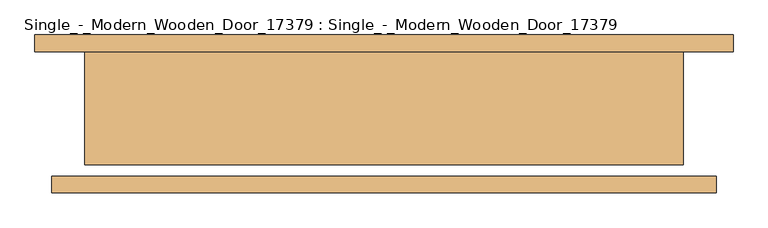
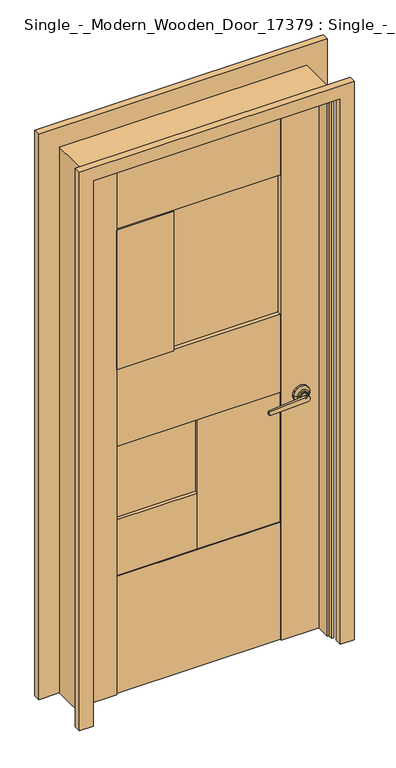
"""IFC4 building model written with IfcOpenShell, lengths in millimetres: door geometry, Single_-_Modern_Wooden_Door_17379 : Single_-_Modern_Wooden_Door_17379."""

from ifc_helpers import new_model, si_unit, point, frame, frame_2d, origin, origin_with_axes, place, context, project, spatial, polyline, circle_curve, ellipse_curve, trimmed, segment, composite_curve, outline, extrude, faceted_brep, source, transform, mapped, element, save
from ifc_brep_helpers import plane_surface, cylinder_surface, revolved_surface, advanced_brep


def single_modern_wooden_door_17379_single_modern_wooden_door_9761f21e(model_context):
    return source(origin(), model_context, "Body", "SolidModel", [
        extrude(outline(polyline([(2133.6, -457.2), (2133.6, 457.2), (0.0, 457.2), (0.0, 508.0), (2184.4, 508.0), (2184.4, -508.0), (0.0, -508.0), (0.0, -457.2), (2133.6, -457.2)])), frame((0.0, -139.7, 0.0), z_axis=(0.0, 1.0, 0.0), x_axis=(0.0, 0.0, 1.0)), (0.0, 0.0, 1.0), 25.4),
        advanced_brep(
        [(533.4, 76.2, 0.0), (457.2, 76.2, 0.0), (457.2, 88.9, 0.0), (479.425, 88.9, 0.0), (479.425, 95.25, 0.0), (485.775, 101.6, 0.0), (533.4, 101.6, 0.0), (533.4, 76.2, 2209.8), (-533.4, 76.2, 2209.8), (-533.4, 76.2, 0.0), (-457.2, 76.2, 0.0), (-457.2, 76.2, 2133.6), (457.2, 76.2, 2133.6), (457.2, 88.9, 2133.6), (-457.2, 88.9, 2133.6), (-457.2, 88.9, 0.0), (-479.425, 88.9, 0.0), (-479.425, 88.9, 2155.825), (479.425, 88.9, 2155.825), (479.425, 95.25, 2155.825), (485.775, 101.6, 2162.175), (-485.775, 101.6, 2162.175), (-485.775, 101.6, 0.0), (-533.4, 101.6, 0.0), (-533.4, 101.6, 2209.8), (533.4, 101.6, 2209.8), (-479.425, 95.25, 0.0), (-479.425, 95.25, 2155.825)],
        [
            (0, 1),
            (1, 2),
            (2, 3),
            (3, 4),
            (4, 5, circle_curve(frame((485.775, 95.25, 0.0), z_axis=(0.0, 0.0, -1.0), x_axis=(-1.0, 0.0, 0.0)), 6.35)),
            (5, 6),
            (6, 0),
            (0, 7),
            (7, 8),
            (8, 9),
            (9, 10),
            (10, 11),
            (11, 12),
            (12, 1),
            (12, 13),
            (13, 2),
            (13, 14),
            (14, 15),
            (15, 16),
            (16, 17),
            (17, 18),
            (18, 3),
            (18, 19),
            (19, 4),
            (19, 20, ellipse_curve(frame((485.775, 95.25, 2162.175), z_axis=(0.7071067811865457, 0.0, -0.7071067811865492), x_axis=(-0.7071067811865492, 0.0, -0.7071067811865458)), 8.9802561, 6.35)),
            (20, 5),
            (20, 21),
            (21, 22),
            (22, 23),
            (23, 24),
            (24, 25),
            (25, 6),
            (25, 7),
            (8, 24),
            (23, 9),
            (22, 26, circle_curve(frame((-485.775, 95.25, 0.0), z_axis=(0.0, 0.0, -1.0), x_axis=(1.0, 0.0, 0.0)), 6.35)),
            (26, 16),
            (15, 10),
            (14, 11),
            (27, 17),
            (26, 27),
            (21, 27, ellipse_curve(frame((-485.775, 95.25, 2162.175), z_axis=(-0.7071067811865492, 0.0, -0.7071067811865458), x_axis=(-0.7071067811865458, 0.0, 0.7071067811865492)), 8.9802561, 6.35)),
            (27, 19),
        ],
        [
            plane_surface(frame((457.2, 0.0, 0.0), z_axis=(0.0, 0.0, -1.0), x_axis=(0.0, -1.0, 0.0))),
            plane_surface(frame((533.4, 76.2, 0.0), z_axis=(0.0, -1.0, 0.0), x_axis=(0.0, 0.0, 1.0))),
            plane_surface(frame((457.2, 76.2, 0.0), z_axis=(-1.0, 0.0, 0.0), x_axis=(0.0, 0.0, 1.0))),
            plane_surface(frame((457.2, 88.9, 0.0), z_axis=(0.0, 1.0, 0.0), x_axis=(0.0, 0.0, 1.0))),
            plane_surface(frame((479.425, 88.9, 0.0), z_axis=(-1.0, 0.0, 0.0), x_axis=(0.0, 0.0, 1.0))),
            cylinder_surface(frame((485.775, 95.25, 0.0), z_axis=(0.0, 0.0, -1.0), x_axis=(-1.0, 0.0, 0.0)), 6.35),
            plane_surface(frame((485.775, 101.6, 0.0), z_axis=(0.0, 1.0, 0.0), x_axis=(0.0, 0.0, 1.0))),
            plane_surface(frame((533.4, 101.6, 0.0), z_axis=(1.0, 0.0, 0.0), x_axis=(0.0, 0.0, 1.0))),
            plane_surface(frame((-533.4, 101.6, 2209.8), z_axis=(-1.0, 0.0, 0.0), x_axis=(0.0, 0.0, -1.0))),
            plane_surface(frame((-457.2, 0.0, 0.0), z_axis=(0.0, 0.0, -1.0), x_axis=(0.0, -1.0, 0.0))),
            plane_surface(frame((-457.2, 76.2, 2133.6), z_axis=(1.0, 0.0, 0.0), x_axis=(0.0, 0.0, -1.0))),
            plane_surface(frame((-479.425, 88.9, 2155.825), z_axis=(1.0, 0.0, 0.0), x_axis=(0.0, 0.0, -1.0))),
            cylinder_surface(frame((-485.775, 95.25, 2133.6), z_axis=(0.0, 0.0, 1.0), x_axis=(1.0, 0.0, 0.0)), 6.35),
            plane_surface(frame((457.2, 76.2, 2133.6), z_axis=(0.0, 0.0, -1.0), x_axis=(-1.0, 0.0, 0.0))),
            plane_surface(frame((479.425, 88.9, 2155.825), z_axis=(0.0, 0.0, -1.0), x_axis=(-1.0, 0.0, 0.0))),
            cylinder_surface(frame((457.2, 95.25, 2162.175), z_axis=(1.0, 0.0, 0.0), x_axis=(0.0, 0.0, -1.0)), 6.35),
            plane_surface(frame((533.4, 101.6, 2209.8), z_axis=(0.0, 0.0, 1.0), x_axis=(-1.0, 0.0, 0.0))),
        ],
        [
            (0, [[1, 2, 3, 4, 5, 6, 7]]),
            (1, [[-1, 8, 9, 10, 11, 12, 13, 14]]),
            (2, [[-2, -14, 15, 16]]),
            (3, [[-3, -16, 17, 18, 19, 20, 21, 22]]),
            (4, [[-4, -22, 23, 24]]),
            (5, [[-5, -24, 25, 26]]),
            (6, [[-6, -26, 27, 28, 29, 30, 31, 32]]),
            (7, [[-7, -32, 33, -8]]),
            (8, [[34, -30, 35, -10]]),
            (9, [[-35, -29, 36, 37, -19, 38, -11]]),
            (10, [[39, -12, -38, -18]]),
            (11, [[40, -20, -37, 41]]),
            (12, [[42, -41, -36, -28]]),
            (13, [[-15, -13, -39, -17]]),
            (14, [[-23, -21, -40, 43]]),
            (15, [[-25, -43, -42, -27]]),
            (16, [[-33, -31, -34, -9]]),
        ],
    ),
        faceted_brep([(444.5, 76.2, 0.0), (457.2, 76.2, 0.0), (457.2, -96.9526688, 0.0), (449.8578125, -96.9526688, 0.0), (449.8578125, -78.3473783, 0.0), (444.5, -78.3473783, 0.0), (444.5, 76.2, 2120.9), (-444.5, 76.2, 2120.9), (-444.5, 76.2, 0.0), (-457.2, 76.2, 0.0), (-457.2, 76.2, 2133.6), (457.2, 76.2, 2133.6), (457.2, -96.9526688, 2133.6), (-457.2, -96.9526688, 2133.6), (-457.2, -96.9526688, 0.0), (-449.8578125, -96.9526688, 0.0), (-449.8578125, -96.9526688, 2126.2578125), (449.8578125, -96.9526688, 2126.2578125), (449.8578125, -78.3473783, 2126.2578125), (-449.8578125, -78.3473783, 2126.2578125), (-449.8578125, -78.3473783, 0.0), (-444.5, -78.3473783, 0.0), (-444.5, -78.3473783, 2120.9), (444.5, -78.3473783, 2120.9)], [[[0, 1, 2, 3, 4, 5]], [[1, 0, 6, 7, 8, 9, 10, 11]], [[2, 1, 11, 12]], [[3, 2, 12, 13, 14, 15, 16, 17]], [[4, 3, 17, 18]], [[5, 4, 18, 19, 20, 21, 22, 23]], [[0, 5, 23, 6]], [[7, 22, 21, 8]], [[8, 21, 20, 15, 14, 9]], [[13, 10, 9, 14]], [[19, 16, 15, 20]], [[12, 11, 10, 13]], [[6, 23, 22, 7]], [[18, 17, 16, 19]]]),
        extrude(outline(polyline([(-304.8, -25.4), (-444.5, -25.4), (-444.5, 25.4), (-304.8, 25.4), (-304.8, -25.4)])), origin_with_axes(), (0.0, 0.0, 1.0), 2120.9),
        extrude(outline(polyline([(444.5, -25.4), (304.8, -25.4), (304.8, 25.4), (444.5, 25.4), (444.5, -25.4)])), origin_with_axes(), (0.0, 0.0, 1.0), 2120.9),
        extrude(outline(polyline([(304.8, -19.05), (-304.8, -19.05), (-304.8, 19.05), (304.8, 19.05), (304.8, -19.05)])), frame((0.0, 0.0, 0.7183756), z_axis=(0.0, 0.0, 1.0), x_axis=(1.0, 0.0, 0.0)), (0.0, 0.0, 1.0), 457.2),
        extrude(outline(polyline([(304.8, -19.05), (-304.8, -19.05), (-304.8, 19.05), (304.8, 19.05), (304.8, -19.05)])), frame((0.0, 0.0, 965.6301148), z_axis=(0.0, 0.0, 1.0), x_axis=(1.0, 0.0, 0.0)), (0.0, 0.0, 1.0), 304.8),
        extrude(outline(polyline([(304.8, -19.05), (-304.8, -19.05), (-304.8, 19.05), (304.8, 19.05), (304.8, -19.05)])), frame((0.0, 0.0, 1816.1), z_axis=(0.0, 0.0, 1.0), x_axis=(1.0, 0.0, 0.0)), (0.0, 0.0, 1.0), 304.8),
        extrude(outline(polyline([(304.8, -2.7903573), (-304.8, -2.7903573), (-304.8, 3.5596427), (304.8, 3.5596427), (304.8, -2.7903573)])), frame((0.0, 0.0, 676.8253621), z_axis=(0.0, 0.0, 1.0), x_axis=(1.0, 0.0, 0.0)), (0.0, 0.0, 1.0), 1139.2746379),
        extrude(outline(polyline([(-93.0839177, -25.4), (-304.8, -25.4), (-304.8, 15.875), (-93.0839177, 15.875), (-93.0839177, -25.4)])), frame((0.0, 0.0, 1270.4301148), z_axis=(0.0, 0.0, 1.0), x_axis=(1.0, 0.0, 0.0)), (0.0, 0.0, 1.0), 545.6698852),
        extrude(outline(polyline([(304.8, -15.875), (0.0, -15.875), (0.0, 15.875), (304.8, 15.875), (304.8, -15.875)])), frame((0.0, 0.0, 457.9183756), z_axis=(0.0, 0.0, 1.0), x_axis=(1.0, 0.0, 0.0)), (0.0, 0.0, 1.0), 507.7117392),
        extrude(outline(polyline([(0.0, -15.875), (-304.8, -15.875), (-304.8, 15.875), (0.0, 15.875), (0.0, -15.875)])), frame((0.0, 0.0, 457.9183756), z_axis=(0.0, 0.0, 1.0), x_axis=(1.0, 0.0, 0.0)), (0.0, 0.0, 1.0), 218.9069865),
        advanced_brep(
        [(344.5942945, 33.3375, 944.6720157), (405.1016039, 33.3375, 944.6720157), (405.1016039, 26.9875, 944.6720157), (344.5942945, 26.9875, 944.6720157), (353.5745507, 42.3177561, 944.6720157), (396.1213477, 42.3177561, 944.6720157), (359.9245507, 42.3177561, 944.6720157), (389.7713477, 42.3177561, 944.6720157), (359.9245507, 48.6677561, 944.6720157), (389.7713477, 48.6677561, 944.6720157), (374.8479492, 48.6677561, 944.6720157), (374.8479492, 26.9875, 944.6720157)],
        [
            (0, 1, circle_curve(frame((374.8479492, 33.3375, 944.6720157), z_axis=(0.0, -1.0, 0.0), x_axis=(1.0, 0.0, 0.0)), 30.2536547)),
            (1, 2),
            (2, 3, circle_curve(frame((374.8479492, 26.9875, 944.6720157), z_axis=(0.0, 1.0, 0.0), x_axis=(1.0, 0.0, 0.0)), 30.2536547)),
            (3, 0),
            (1, 0, circle_curve(frame((374.8479492, 33.3375, 944.6720157), z_axis=(0.0, -1.0, 0.0), x_axis=(1.0, 0.0, 0.0)), 30.2536547)),
            (3, 2, circle_curve(frame((374.8479492, 26.9875, 944.6720157), z_axis=(0.0, 1.0, 0.0), x_axis=(1.0, 0.0, 0.0)), 30.2536547)),
            (4, 5, circle_curve(frame((374.8479492, 42.3177561, 944.6720157), z_axis=(0.0, -1.0, 0.0), x_axis=(1.0, 0.0, 0.0)), 21.2733985)),
            (5, 1),
            (0, 4),
            (5, 4, circle_curve(frame((374.8479492, 42.3177561, 944.6720157), z_axis=(0.0, -1.0, 0.0), x_axis=(1.0, 0.0, 0.0)), 21.2733985)),
            (6, 7, circle_curve(frame((374.8479492, 42.3177561, 944.6720157), z_axis=(0.0, -1.0, 0.0), x_axis=(1.0, 0.0, 0.0)), 14.9233985)),
            (7, 5),
            (4, 6),
            (7, 6, circle_curve(frame((374.8479492, 42.3177561, 944.6720157), z_axis=(0.0, -1.0, 0.0), x_axis=(1.0, 0.0, 0.0)), 14.9233985)),
            (8, 9, circle_curve(frame((374.8479492, 48.6677561, 944.6720157), z_axis=(0.0, -1.0, 0.0), x_axis=(1.0, 0.0, 0.0)), 14.9233985)),
            (9, 7),
            (6, 8),
            (9, 8, circle_curve(frame((374.8479492, 48.6677561, 944.6720157), z_axis=(0.0, -1.0, 0.0), x_axis=(1.0, 0.0, 0.0)), 14.9233985)),
            (10, 9),
            (8, 10),
            (2, 11),
            (11, 3),
        ],
        [
            cylinder_surface(frame((374.8479492, 26.9875, 944.6720157), z_axis=(0.0, 1.0, 0.0), x_axis=(1.0, 0.0, 0.0)), 30.2536547),
            revolved_surface(polyline([(405.1016039, 33.3375, 944.6720157), (396.1213477, 42.3177561, 944.6720157)]), (374.8479492, 26.9875, 944.6720157), (0.0, 1.0, 0.0)),
            plane_surface(frame((374.8479492, 42.3177561, 944.6720157), z_axis=(0.0, 1.0, 0.0), x_axis=(1.0, 0.0, 0.0))),
            cylinder_surface(frame((374.8479492, 26.9875, 944.6720157), z_axis=(0.0, 1.0, 0.0), x_axis=(1.0, 0.0, 0.0)), 14.9233985),
            plane_surface(frame((374.8479492, 48.6677561, 944.6720157), z_axis=(0.0, 1.0, 0.0), x_axis=(1.0, 0.0, 0.0))),
            plane_surface(frame((374.8479492, 26.9875, 944.6720157), z_axis=(0.0, -1.0, 0.0), x_axis=(1.0, 0.0, 0.0))),
        ],
        [
            (0, [[1, 2, 3, 4]]),
            (0, [[5, -4, 6, -2]]),
            (1, [[7, 8, -1, 9]]),
            (1, [[10, -9, -5, -8]]),
            (2, [[11, 12, -7, 13]]),
            (2, [[14, -13, -10, -12]]),
            (3, [[15, 16, -11, 17]]),
            (3, [[18, -17, -14, -16]]),
            (4, [[19, -15, 20]]),
            (4, [[-20, -18, -19]]),
            (5, [[-3, 21, 22]]),
            (5, [[-6, -22, -21]]),
        ],
    ),
        extrude(outline(composite_curve([segment(trimmed(circle_curve(frame_2d((945.0636166, 375.0281858)), 10.5195008), [point((945.0636166, 364.508685))], [point((945.0636166, 385.5476866))], False, "CARTESIAN"), True, "CONTINUOUS"), segment(trimmed(circle_curve(frame_2d((945.0636166, 375.0281858)), 10.5195008), [point((945.0636166, 385.5476866))], [point((945.0636166, 364.508685))], False, "CARTESIAN"), True, "CONTINUOUS")], self_intersect=False)), frame((0.0, 48.6677561, 0.0), z_axis=(0.0, 1.0, 0.0), x_axis=(0.0, 0.0, 1.0)), (0.0, 0.0, 1.0), 12.7),
        extrude(outline(composite_curve([segment(trimmed(circle_curve(frame_2d((944.8067047, 374.8708472)), 10.5195008), [point((934.3128289, 375.6046505))], [point((955.3005805, 374.1370439))], False, "CARTESIAN"), True, "CONTINUOUS"), segment(polyline([(955.3005805, 374.1370439), (941.7771559, 235.0415607), (929.1080925, 235.927468), (934.3128289, 375.6046505)]), True, "CONTINUOUS")], self_intersect=False)), frame((0.0, 61.3677561, 0.0), z_axis=(0.0, 1.0, 0.0), x_axis=(0.0, 0.0, 1.0)), (0.0, 0.0, 1.0), 7.9400683),
        extrude(outline(composite_curve([segment(trimmed(circle_curve(frame_2d((889.0183611, 374.8479492)), 9.8730778), [point((889.0183611, 364.9748714))], [point((889.0183611, 384.721027))], False, "CARTESIAN"), True, "CONTINUOUS"), segment(trimmed(circle_curve(frame_2d((889.0183611, 374.8479492)), 9.8730778), [point((889.0183611, 384.721027))], [point((889.0183611, 364.9748714))], False, "CARTESIAN"), True, "CONTINUOUS")], self_intersect=False)), frame((0.0, 25.4, 0.0), z_axis=(0.0, 1.0, 0.0), x_axis=(0.0, 0.0, 1.0)), (0.0, 0.0, 1.0), 7.9375),
        advanced_brep(
        [(344.5942945, -26.9875, 944.6720157), (405.1016039, -26.9875, 944.6720157), (405.1016039, -33.3375, 944.6720157), (344.5942945, -33.3375, 944.6720157), (396.1213477, -42.3177561, 944.6720157), (353.5745507, -42.3177561, 944.6720157), (389.7713477, -42.3177561, 944.6720157), (359.9245507, -42.3177561, 944.6720157), (389.7713477, -48.6677561, 944.6720157), (359.9245507, -48.6677561, 944.6720157), (374.8479492, -48.6677561, 944.6720157), (374.8479492, -26.9875, 944.6720157)],
        [
            (0, 1, circle_curve(frame((374.8479492, -26.9875, 944.6720157), z_axis=(0.0, -1.0, 0.0), x_axis=(1.0, 0.0, 0.0)), 30.2536547)),
            (1, 2),
            (2, 3, circle_curve(frame((374.8479492, -33.3375, 944.6720157), z_axis=(0.0, 1.0, 0.0), x_axis=(1.0, 0.0, 0.0)), 30.2536547)),
            (3, 0),
            (1, 0, circle_curve(frame((374.8479492, -26.9875, 944.6720157), z_axis=(0.0, -1.0, 0.0), x_axis=(1.0, 0.0, 0.0)), 30.2536547)),
            (3, 2, circle_curve(frame((374.8479492, -33.3375, 944.6720157), z_axis=(0.0, 1.0, 0.0), x_axis=(1.0, 0.0, 0.0)), 30.2536547)),
            (2, 4),
            (4, 5, circle_curve(frame((374.8479492, -42.3177561, 944.6720157), z_axis=(0.0, 1.0, 0.0), x_axis=(1.0, 0.0, 0.0)), 21.2733985)),
            (5, 3),
            (5, 4, circle_curve(frame((374.8479492, -42.3177561, 944.6720157), z_axis=(0.0, 1.0, 0.0), x_axis=(1.0, 0.0, 0.0)), 21.2733985)),
            (4, 6),
            (6, 7, circle_curve(frame((374.8479492, -42.3177561, 944.6720157), z_axis=(0.0, 1.0, 0.0), x_axis=(1.0, 0.0, 0.0)), 14.9233985)),
            (7, 5),
            (7, 6, circle_curve(frame((374.8479492, -42.3177561, 944.6720157), z_axis=(0.0, 1.0, 0.0), x_axis=(1.0, 0.0, 0.0)), 14.9233985)),
            (6, 8),
            (8, 9, circle_curve(frame((374.8479492, -48.6677561, 944.6720157), z_axis=(0.0, 1.0, 0.0), x_axis=(1.0, 0.0, 0.0)), 14.9233985)),
            (9, 7),
            (9, 8, circle_curve(frame((374.8479492, -48.6677561, 944.6720157), z_axis=(0.0, 1.0, 0.0), x_axis=(1.0, 0.0, 0.0)), 14.9233985)),
            (8, 10),
            (10, 9),
            (11, 1),
            (0, 11),
        ],
        [
            cylinder_surface(frame((374.8479492, -26.9875, 944.6720157), z_axis=(0.0, 1.0, 0.0), x_axis=(1.0, 0.0, 0.0)), 30.2536547),
            revolved_surface(polyline([(396.1213477, -42.3177561, 944.6720157), (405.1016039, -33.3375, 944.6720157)]), (374.8479492, -26.9875, 944.6720157), (0.0, 1.0, 0.0)),
            plane_surface(frame((374.8479492, -42.3177561, 944.6720157), z_axis=(0.0, -1.0, 0.0), x_axis=(1.0, 0.0, 0.0))),
            cylinder_surface(frame((374.8479492, -26.9875, 944.6720157), z_axis=(0.0, 1.0, 0.0), x_axis=(1.0, 0.0, 0.0)), 14.9233985),
            plane_surface(frame((374.8479492, -48.6677561, 944.6720157), z_axis=(0.0, -1.0, 0.0), x_axis=(1.0, 0.0, 0.0))),
            plane_surface(frame((374.8479492, -26.9875, 944.6720157), z_axis=(0.0, 1.0, 0.0), x_axis=(1.0, 0.0, 0.0))),
        ],
        [
            (0, [[1, 2, 3, 4]]),
            (0, [[5, -4, 6, -2]]),
            (1, [[-3, 7, 8, 9]]),
            (1, [[-6, -9, 10, -7]]),
            (2, [[-8, 11, 12, 13]]),
            (2, [[-10, -13, 14, -11]]),
            (3, [[-12, 15, 16, 17]]),
            (3, [[-14, -17, 18, -15]]),
            (4, [[-16, 19, 20]]),
            (4, [[-18, -20, -19]]),
            (5, [[21, -1, 22]]),
            (5, [[-22, -5, -21]]),
        ],
    ),
        extrude(outline(composite_curve([segment(trimmed(circle_curve(frame_2d((945.0636166, 375.0281858)), 10.5195008), [point((945.0636166, 364.508685))], [point((945.0636166, 385.5476866))], False, "CARTESIAN"), True, "CONTINUOUS"), segment(trimmed(circle_curve(frame_2d((945.0636166, 375.0281858)), 10.5195008), [point((945.0636166, 385.5476866))], [point((945.0636166, 364.508685))], False, "CARTESIAN"), True, "CONTINUOUS")], self_intersect=False)), frame((0.0, 48.6677561, 0.0), z_axis=(0.0, 1.0, 0.0), x_axis=(0.0, 0.0, 1.0)), (0.0, 0.0, 1.0), 12.7),
        extrude(outline(composite_curve([segment(trimmed(circle_curve(frame_2d((944.8067047, 375.0459405)), 10.5195008), [point((934.3253704, 375.9412215))], [point((955.3005805, 374.3121372))], False, "CARTESIAN"), True, "CONTINUOUS"), segment(polyline([(955.3005805, 374.3121372), (941.7771559, 235.0415607), (929.1080925, 235.927468), (934.3253704, 375.9412215)]), True, "CONTINUOUS")], self_intersect=False)), frame((0.0, 61.3677561, 0.0), z_axis=(0.0, 1.0, 0.0), x_axis=(0.0, 0.0, 1.0)), (0.0, 0.0, 1.0), 7.9400683),
        extrude(outline(composite_curve([segment(trimmed(circle_curve(frame_2d((945.0636166, 375.3374053)), 10.5195008), [point((945.0636166, 385.8569061))], [point((945.0636166, 364.8179045))], False, "CARTESIAN"), True, "CONTINUOUS"), segment(trimmed(circle_curve(frame_2d((945.0636166, 375.3374053)), 10.5195008), [point((945.0636166, 364.8179045))], [point((945.0636166, 385.8569061))], False, "CARTESIAN"), True, "CONTINUOUS")], self_intersect=False)), frame((0.0, -61.3677561, 0.0), z_axis=(0.0, 1.0, 0.0), x_axis=(0.0, 0.0, 1.0)), (0.0, 0.0, 1.0), 12.7),
        extrude(outline(composite_curve([segment(trimmed(circle_curve(frame_2d((944.8067047, 375.2983948)), 10.5195008), [point((934.3253704, 376.1936758))], [point((955.3005805, 374.5645915))], False, "CARTESIAN"), True, "CONTINUOUS"), segment(polyline([(955.3005805, 374.5645915), (941.7771559, 235.2940151), (929.1080925, 236.1799223), (934.3253704, 376.1936758)]), True, "CONTINUOUS")], self_intersect=False)), frame((0.0, -69.336388, 0.0), z_axis=(0.0, 1.0, 0.0), x_axis=(0.0, 0.0, 1.0)), (0.0, 0.0, 1.0), 7.9400683),
    ])


if __name__ == "__main__":
    model = new_model("IFC4")
    model_context = context("Model", 3, world=origin())
    ifc_project = project(units=[si_unit("LENGTHUNIT", "METRE", prefix="MILLI")], contexts=[model_context])
    site = spatial("IfcSite", under=ifc_project)
    building = spatial("IfcBuilding", under=site)
    placement = place(None, origin())
    single_modern_wooden_door_17379_single_modern_wooden_door_shape = single_modern_wooden_door_17379_single_modern_wooden_door_9761f21e(model_context)
    element("IfcDoor", 1, ObjectType="Single_-_Modern_Wooden_Door_17379 : Single_-_Modern_Wooden_Door_17379", at=placement, inside=building, context=model_context, shape_type="MappedRepresentation", body=[
        mapped(single_modern_wooden_door_17379_single_modern_wooden_door_shape, transform((0.0, 0.0, 0.0), x_axis=(1.0, 0.0, 0.0), y_axis=(0.0, 1.0, 0.0), z_axis=(0.0, 0.0, 1.0))),
    ])
    save(model, "model.ifc")

# Revit data of these elements
# Type "Single_-_Modern_Wooden_Door_17379 : Single_-_Modern_Wooden_Door_17379"
#   Type Mark = "8"
#   Frame Projection Ext. = 0' - 1"
#   Frame Projection Int. = 0' - 1"
#   Frame Width = 0' - 2"
#   Height = 7' - 0"
#   Width = 3' - 0"
#   Handel = Stainless Steel AISI 304
#   Glass = Glass
#   Door Frame = Wood (Oak)
#   Door = Custom Walnut
#   Function = (empty or 0)
#   Wall Closure = (empty or 0)
# Element 1 (IfcDoor, "Single_-_Modern_Wooden_Door_17379 : Single_-_Modern_Wooden_Door_17379")
#   Materials on its faces: "Stainless Steel AISI 304", "Custom Walnut", "Wood (Oak)", "Glass"
# Materials
#   "Stainless Steel AISI 304": class "Metal", colour RGB 244 244 244, transparency 0, Description = "Stainless Steel 18/8", Cost = 0
#   "Glass": class "Glass", colour RGB 0 128 192, transparency 0.75, Description = "Soda Lime Glass", Cost = 0
#   "Wood (Oak)": class "Wood", colour RGB 132 88 61, transparency 0, Description = "Physical material.", Cost = 0
#   "Custom Walnut": class "Wood", colour RGB 95 44 25, transparency 0, Description = "Juglans Nigra", Cost = 0
